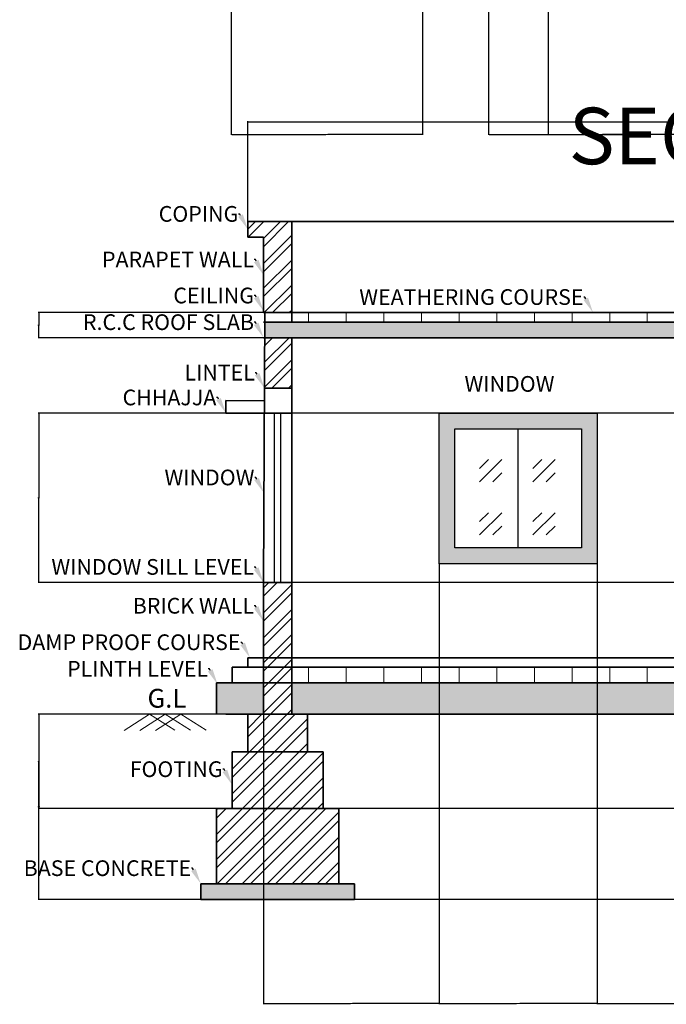
# Model space of a CAD drawing. Units: inches. Extents: x -301 to 715, y -607 to 364.
# Tile 1 of 141: x -272 to -66, y -574 to -260. Entities that reach past the tile are written whole.
import ezdxf
from ezdxf import colors
from ezdxf.entities.mleader import LeaderData, LeaderLine
from ezdxf.math import Vec2, Vec3

# ---------------------------------------------------------------- set-up
doc = ezdxf.new("R2010")
doc.units = ezdxf.units.IN
doc.header["$MEASUREMENT"] = 0
for name, color, linetype, lineweight in [('A-ANNO-DIMS', 2, 'Continuous', 18), ('A-ANNO-SYMB', 4, 'Continuous', 18), ('A-ANNO-TEXT', 4, 'Continuous', 18), ('A-ANNO-TITL', 1, 'Continuous', 35), ('A-GLAZ', 2, 'Continuous', 25), ('A-GRND', 7, 'Continuous', 25), ('A-SECT', 1, 'Continuous', 35), ('A-SECT-PATT', 8, 'Continuous', 13), ('S-FNDN', 2, 'Continuous', 35)]:
    doc.layers.add(name, color=color, linetype=linetype, lineweight=lineweight)
doc.styles.get("Standard").update_dxf_attribs({"font": 'arial.ttf'})
doc.dimstyles.get("Standard").update_dxf_attribs({"dimtxt": 0.18, "dimasz": 0.18, "dimexe": 0.18, "dimexo": 0.0625, "dimgap": 0.09, "dimtad": 0, "dimtih": 1, "dimtoh": 1, "dimdec": 1, "dimzin": 0, "dimdsep": 46, "dimlunit": 4, "dimtxsty": 'Standard', "dimcen": 0.09, "dimclrd": 3, "dimclre": 4, "dimclrt": 6, "dimadec": 0, "dimazin": 0, "dimtfac": 1, "dimtdec": 1, "dimtofl": 0, "dimtmove": 0, "dimatfit": 3, "dimfxl": 1, "dimtfill": 2, "dimtfillclr": 51, "dimtolj": 1, "dimtzin": 0, "dimarcsym": 0})

# ---------------------------------------------------------------- blocks, each defined once
blk = doc.blocks.new('GRADE-MARK-3')
for p, q in [((8.05, 5.16), (0, 0)), ((13.05, 5.16), (5, 0)), ((8.05, 5.16), (16.2, 0.15)), ((18.05, 5.16), (10, 0)), ((13.05, 5.16), (21.2, 0.15)), ((18.05, 5.16), (26.2, 0.15))]:
    blk.add_line(p, q)
blk = doc.blocks.new('*D146')
at = {"layer": 'A-ANNO-DIMS', "color": 4, "lineweight": -2, "transparency": 16777216}
for p, q in [((-204.6, -223.88), (-204.6, -296.87)), ((-143.6, -223.88), (-143.6, -296.87))]:
    blk.add_line(p, q, dxfattribs=at)
at = {"layer": 'A-ANNO-DIMS', "color": 3, "lineweight": -2, "transparency": 16777216}
for p, q in [((-204.42, -296.69), (-174.43, -296.69)), ((-143.78, -296.69), (-173.77, -296.69))]:
    blk.add_line(p, q, dxfattribs=at)
at = {"layer": 'A-ANNO-DIMS', "color": 3, "transparency": 16777216}
for points in [[(-204.42, -296.66), (-204.42, -296.72), (-204.6, -296.69)], [(-143.78, -296.66), (-143.78, -296.72), (-143.6, -296.69)]]:
    blk.add_solid(points, dxfattribs=at)
at = {"layer": 'Defpoints', "color": 0, "transparency": 16777216}
for p in [(-204.6, -223.82), (-143.6, -223.82), (-143.6, -296.69)]:
    blk.add_point(p, dxfattribs=at)
at = {"layer": 'A-ANNO-DIMS', "color": 6, "transparency": 16777216, "insert": (-174.1, -296.69), "char_height": 0.18, "attachment_point": 5, "bg_fill": 1, "box_fill_scale": 1.25, "bg_fill_color": 51, "bg_fill_transparency": 0}
blk.add_mtext('\\A1;5\'-1"', dxfattribs=at)
blk = doc.blocks.new('*D147')
at = {"layer": 'A-ANNO-DIMS', "color": 4, "lineweight": -2, "transparency": 16777216}
for p, q in [((-103.6, -223.88), (-103.6, -296.87)), ((-45.6, -223.88), (-45.6, -296.87))]:
    blk.add_line(p, q, dxfattribs=at)
at = {"layer": 'A-ANNO-DIMS', "color": 3, "lineweight": -2, "transparency": 16777216}
for p, q in [((-103.42, -296.69), (-75.01, -296.69)), ((-45.78, -296.69), (-74.2, -296.69))]:
    blk.add_line(p, q, dxfattribs=at)
at = {"layer": 'A-ANNO-DIMS', "color": 3, "transparency": 16777216}
for points in [[(-103.42, -296.66), (-103.42, -296.72), (-103.6, -296.69)], [(-45.78, -296.66), (-45.78, -296.72), (-45.6, -296.69)]]:
    blk.add_solid(points, dxfattribs=at)
at = {"layer": 'Defpoints', "color": 0, "transparency": 16777216}
for p in [(-103.6, -223.82), (-45.6, -223.82), (-45.6, -296.69)]:
    blk.add_point(p, dxfattribs=at)
at = {"layer": 'A-ANNO-DIMS', "color": 6, "transparency": 16777216, "insert": (-74.6, -296.69), "char_height": 0.18, "attachment_point": 5, "bg_fill": 1, "box_fill_scale": 1.25, "bg_fill_color": 51, "bg_fill_transparency": 0}
blk.add_mtext('\\A1;4\'-10"', dxfattribs=at)
blk = doc.blocks.new('*D158')
at = {"layer": 'A-ANNO-DIMS', "color": 4, "lineweight": -2, "transparency": 16777216}
for p, q in [((-122.6, 221.62), (-122.6, -296.87)), ((-50.6, 221.62), (-50.6, -296.87))]:
    blk.add_line(p, q, dxfattribs=at)
at = {"layer": 'A-ANNO-DIMS', "color": 3, "lineweight": -2, "transparency": 16777216}
for p, q in [((-122.42, -296.69), (-86.93, -296.69)), ((-50.78, -296.69), (-86.27, -296.69))]:
    blk.add_line(p, q, dxfattribs=at)
at = {"layer": 'A-ANNO-DIMS', "color": 3, "transparency": 16777216}
for points in [[(-122.42, -296.66), (-122.42, -296.72), (-122.6, -296.69)], [(-50.78, -296.66), (-50.78, -296.72), (-50.6, -296.69)]]:
    blk.add_solid(points, dxfattribs=at)
at = {"layer": 'Defpoints', "color": 0, "transparency": 16777216}
for p in [(-122.6, 221.68), (-50.6, 221.68), (-50.6, -296.69)]:
    blk.add_point(p, dxfattribs=at)
at = {"layer": 'A-ANNO-DIMS', "color": 6, "transparency": 16777216, "insert": (-86.6, -296.69), "char_height": 0.18, "attachment_point": 5, "bg_fill": 1, "box_fill_scale": 1.25, "bg_fill_color": 51, "bg_fill_transparency": 0}
blk.add_mtext('\\A1;6\'-0"', dxfattribs=at)
blk = doc.blocks.new('*D175')
at = {"layer": 'A-ANNO-DIMS', "color": 4, "lineweight": -2, "transparency": 16777216}
for p, q in [((-199.28, -324.41), (-199.28, -292.47)), ((148.22, -324.41), (148.22, -292.47))]:
    blk.add_line(p, q, dxfattribs=at)
at = {"layer": 'A-ANNO-DIMS', "color": 3, "lineweight": -2, "transparency": 16777216}
for p, q in [((-199.1, -292.65), (-26.21, -292.65)), ((148.04, -292.65), (-24.85, -292.65))]:
    blk.add_line(p, q, dxfattribs=at)
at = {"layer": 'A-ANNO-DIMS', "color": 3, "transparency": 16777216}
for points in [[(-199.1, -292.62), (-199.1, -292.68), (-199.28, -292.65)], [(148.04, -292.62), (148.04, -292.68), (148.22, -292.65)]]:
    blk.add_solid(points, dxfattribs=at)
at = {"layer": 'Defpoints', "color": 0, "transparency": 16777216}
for p in [(148.22, -292.65), (-199.28, -324.48), (148.22, -324.48)]:
    blk.add_point(p, dxfattribs=at)
at = {"layer": 'A-ANNO-DIMS', "color": 6, "transparency": 16777216, "insert": (-25.53, -292.65), "char_height": 0.18, "attachment_point": 5, "bg_fill": 1, "box_fill_scale": 1.25, "bg_fill_color": 51, "bg_fill_transparency": 0}
blk.add_mtext('\\A1;28\'-11 1/2"', dxfattribs=at)
blk = doc.blocks.new('*D177')
at = {"layer": 'A-ANNO-DIMS', "color": 4, "lineweight": -2, "transparency": 16777216}
for p, q in [((-138.28, -433.54), (-138.28, -573.81)), ((-194.28, -481.54), (-194.28, -573.81))]:
    blk.add_line(p, q, dxfattribs=at)
at = {"layer": 'A-ANNO-DIMS', "color": 3, "lineweight": -2, "transparency": 16777216}
for p, q in [((-194.1, -573.63), (-166.61, -573.63)), ((-138.46, -573.63), (-165.95, -573.63))]:
    blk.add_line(p, q, dxfattribs=at)
at = {"layer": 'A-ANNO-DIMS', "color": 3, "transparency": 16777216}
for points in [[(-194.1, -573.6), (-194.1, -573.66), (-194.28, -573.63)], [(-138.46, -573.6), (-138.46, -573.66), (-138.28, -573.63)]]:
    blk.add_solid(points, dxfattribs=at)
at = {"layer": 'Defpoints', "color": 0, "transparency": 16777216}
for p in [(-138.28, -433.48), (-194.28, -481.48), (-138.28, -573.63)]:
    blk.add_point(p, dxfattribs=at)
at = {"layer": 'A-ANNO-DIMS', "color": 6, "transparency": 16777216, "insert": (-166.28, -573.63), "char_height": 0.18, "attachment_point": 5, "bg_fill": 1, "box_fill_scale": 1.25, "bg_fill_color": 51, "bg_fill_transparency": 0}
blk.add_mtext('\\A1;4\'-8"', dxfattribs=at)
blk = doc.blocks.new('*D178')
at = {"layer": 'A-ANNO-DIMS', "color": 4, "lineweight": -2, "transparency": 16777216}
for p, q in [((-138.28, -433.54), (-138.28, -573.81)), ((-87.98, -433.54), (-87.98, -573.81))]:
    blk.add_line(p, q, dxfattribs=at)
at = {"layer": 'A-ANNO-DIMS', "color": 3, "lineweight": -2, "transparency": 16777216}
for p, q in [((-138.1, -573.63), (-113.67, -573.63)), ((-88.16, -573.63), (-112.59, -573.63))]:
    blk.add_line(p, q, dxfattribs=at)
at = {"layer": 'A-ANNO-DIMS', "color": 3, "transparency": 16777216}
for points in [[(-138.1, -573.6), (-138.1, -573.66), (-138.28, -573.63)], [(-88.16, -573.6), (-88.16, -573.66), (-87.98, -573.63)]]:
    blk.add_solid(points, dxfattribs=at)
at = {"layer": 'Defpoints', "color": 0, "transparency": 16777216}
for p in [(-138.28, -433.48), (-87.98, -433.48), (-87.98, -573.63)]:
    blk.add_point(p, dxfattribs=at)
at = {"layer": 'A-ANNO-DIMS', "color": 6, "transparency": 16777216, "insert": (-113.13, -573.63), "char_height": 0.18, "attachment_point": 5, "bg_fill": 1, "box_fill_scale": 1.25, "bg_fill_color": 51, "bg_fill_transparency": 0}
blk.add_mtext('\\A1;4\'-2 1/2"', dxfattribs=at)
blk = doc.blocks.new('*D179')
at = {"layer": 'A-ANNO-DIMS', "color": 4, "lineweight": -2, "transparency": 16777216}
for p, q in [((-87.98, -433.54), (-87.98, -573.81)), ((-35.28, -463.54), (-35.28, -573.81))]:
    blk.add_line(p, q, dxfattribs=at)
at = {"layer": 'A-ANNO-DIMS', "color": 3, "lineweight": -2, "transparency": 16777216}
for p, q in [((-87.8, -573.63), (-62.17, -573.63)), ((-35.46, -573.63), (-61.09, -573.63))]:
    blk.add_line(p, q, dxfattribs=at)
at = {"layer": 'A-ANNO-DIMS', "color": 3, "transparency": 16777216}
for points in [[(-87.8, -573.6), (-87.8, -573.66), (-87.98, -573.63)], [(-35.46, -573.6), (-35.46, -573.66), (-35.28, -573.63)]]:
    blk.add_solid(points, dxfattribs=at)
at = {"layer": 'Defpoints', "color": 0, "transparency": 16777216}
for p in [(-87.98, -433.48), (-35.28, -463.48), (-35.28, -573.63)]:
    blk.add_point(p, dxfattribs=at)
at = {"layer": 'A-ANNO-DIMS', "color": 6, "transparency": 16777216, "insert": (-61.63, -573.63), "char_height": 0.18, "attachment_point": 5, "bg_fill": 1, "box_fill_scale": 1.25, "bg_fill_color": 51, "bg_fill_transparency": 0}
blk.add_mtext('\\A1;4\'-4 1/2"', dxfattribs=at)
blk = doc.blocks.new('*D187')
at = {"layer": 'A-ANNO-DIMS', "color": 4, "lineweight": -2, "transparency": 16777216}
for p, q in [((139.67, -385.48), (-266.11, -385.48)), ((143.16, -439.48), (-266.11, -439.48))]:
    blk.add_line(p, q, dxfattribs=at)
at = {"layer": 'A-ANNO-DIMS', "color": 3, "lineweight": -2, "transparency": 16777216}
for p, q in [((-265.93, -385.66), (-265.93, -412.3)), ((-265.93, -439.3), (-265.93, -412.66))]:
    blk.add_line(p, q, dxfattribs=at)
at = {"layer": 'A-ANNO-DIMS', "color": 3, "transparency": 16777216}
for points in [[(-265.96, -385.66), (-265.9, -385.66), (-265.93, -385.48)], [(-265.96, -439.3), (-265.9, -439.3), (-265.93, -439.48)]]:
    blk.add_solid(points, dxfattribs=at)
at = {"layer": 'Defpoints', "color": 0, "transparency": 16777216}
for p in [(-265.93, -385.48), (139.74, -385.48), (143.22, -439.48)]:
    blk.add_point(p, dxfattribs=at)
at = {"layer": 'A-ANNO-DIMS', "color": 6, "transparency": 16777216, "insert": (-265.93, -412.48), "char_height": 0.18, "attachment_point": 5, "bg_fill": 1, "box_fill_scale": 1.25, "bg_fill_color": 51, "bg_fill_transparency": 0}
blk.add_mtext('\\A1;4\'-6"', dxfattribs=at)
blk = doc.blocks.new('*D189')
at = {"layer": 'A-ANNO-DIMS', "color": 4, "lineweight": -2, "transparency": 16777216}
for p, q in [((134.19, -353.48), (-266.11, -353.48)), ((134.19, -361.48), (-266.11, -361.48))]:
    blk.add_line(p, q, dxfattribs=at)
at = {"layer": 'A-ANNO-DIMS', "color": 3, "lineweight": -2, "transparency": 16777216}
for p, q in [((-265.93, -353.66), (-265.93, -357.3)), ((-265.93, -361.3), (-265.93, -357.66))]:
    blk.add_line(p, q, dxfattribs=at)
at = {"layer": 'A-ANNO-DIMS', "color": 3, "transparency": 16777216}
for points in [[(-265.96, -353.66), (-265.9, -353.66), (-265.93, -353.48)], [(-265.96, -361.3), (-265.9, -361.3), (-265.93, -361.48)]]:
    blk.add_solid(points, dxfattribs=at)
at = {"layer": 'Defpoints', "color": 0, "transparency": 16777216}
for p in [(134.26, -353.48), (-265.93, -361.48), (134.26, -361.48)]:
    blk.add_point(p, dxfattribs=at)
at = {"layer": 'A-ANNO-DIMS', "color": 6, "transparency": 16777216, "insert": (-265.93, -357.48), "char_height": 0.18, "attachment_point": 5, "bg_fill": 1, "box_fill_scale": 1.25, "bg_fill_color": 51, "bg_fill_transparency": 0}
blk.add_mtext('\\A1;0\'-8"', dxfattribs=at)
blk = doc.blocks.new('*D190')
at = {"layer": 'A-ANNO-DIMS', "color": 4, "lineweight": -2, "transparency": 16777216}
for p, q in [((129.19, -481.48), (-266.11, -481.48)), ((124.19, -511.48), (-266.11, -511.48))]:
    blk.add_line(p, q, dxfattribs=at)
at = {"layer": 'A-ANNO-DIMS', "color": 3, "lineweight": -2, "transparency": 16777216}
for p, q in [((-265.93, -481.66), (-265.93, -496.3)), ((-265.93, -511.3), (-265.93, -496.66))]:
    blk.add_line(p, q, dxfattribs=at)
at = {"layer": 'A-ANNO-DIMS', "color": 3, "transparency": 16777216}
for points in [[(-265.96, -481.66), (-265.9, -481.66), (-265.93, -481.48)], [(-265.96, -511.3), (-265.9, -511.3), (-265.93, -511.48)]]:
    blk.add_solid(points, dxfattribs=at)
at = {"layer": 'Defpoints', "color": 0, "transparency": 16777216}
for p in [(129.26, -481.48), (-265.93, -511.48), (124.26, -511.48)]:
    blk.add_point(p, dxfattribs=at)
at = {"layer": 'A-ANNO-DIMS', "color": 6, "transparency": 16777216, "insert": (-265.93, -496.48), "char_height": 0.18, "attachment_point": 5, "bg_fill": 1, "box_fill_scale": 1.25, "bg_fill_color": 51, "bg_fill_transparency": 0}
blk.add_mtext('\\A1;2\'-6"', dxfattribs=at)
blk = doc.blocks.new('*D191')
at = {"layer": 'A-ANNO-DIMS', "color": 4, "lineweight": -2, "transparency": 16777216}
for p, q in [((129.19, -481.48), (-266.11, -481.48)), ((114.19, -540.48), (-266.11, -540.48))]:
    blk.add_line(p, q, dxfattribs=at)
at = {"layer": 'A-ANNO-DIMS', "color": 3, "lineweight": -2, "transparency": 16777216}
for p, q in [((-265.93, -481.66), (-265.93, -510.8)), ((-265.93, -540.3), (-265.93, -511.16))]:
    blk.add_line(p, q, dxfattribs=at)
at = {"layer": 'A-ANNO-DIMS', "color": 3, "transparency": 16777216}
for points in [[(-265.96, -481.66), (-265.9, -481.66), (-265.93, -481.48)], [(-265.96, -540.3), (-265.9, -540.3), (-265.93, -540.48)]]:
    blk.add_solid(points, dxfattribs=at)
at = {"layer": 'Defpoints', "color": 0, "transparency": 16777216}
for p in [(129.26, -481.48), (-265.93, -540.48), (114.26, -540.48)]:
    blk.add_point(p, dxfattribs=at)
at = {"layer": 'A-ANNO-DIMS', "color": 6, "transparency": 16777216, "insert": (-265.93, -510.98), "char_height": 0.18, "attachment_point": 5, "bg_fill": 1, "box_fill_scale": 1.25, "bg_fill_color": 51, "bg_fill_transparency": 0}
blk.add_mtext('\\A1;4\'-11"', dxfattribs=at)

msp = doc.modelspace()

# ---------------------------------------------------------------- hatches: boundary and pattern name
at = {"layer": 'A-SECT-PATT'}
h = msp.add_hatch(dxfattribs=at)
h.set_pattern_fill('ANSI32', color=256, scale=15)
h.set_pattern_definition([(45, (10.321, 33.8764), (-3.977476, 3.977476), []), (45, (12.973, 33.8764), (-3.977476, 3.977476), [])])
h.paths.add_polyline_path([(-185.28, -324.48), (-199.28, -324.48), (-199.28, -329.48), (-194.28, -329.48), (-194.28, -353.48), (-185.28, -353.48)])
h.paths.add_polyline_path([(-185.28, -361.48), (-193.9, -361.48), (-193.98, -377.54), (-185.28, -377.54)])
h.paths.add_polyline_path([(143.22, -329.48), (148.22, -329.48), (148.22, -324.48), (134.26, -324.48), (134.26, -353.48), (143.22, -353.48)])
h.paths.add_polyline_path([(143.22, -361.48), (134.26, -361.48), (134.26, -377.48), (143.22, -377.48)])
h.paths.add_polyline_path([(-185.28, -439.48), (-194.28, -439.48), (-194.28, -463.48), (-185.28, -463.48)])
h.paths.add_polyline_path([(-185.28, -471.48), (-194.28, -471.48), (-194.28, -481.48), (-185.28, -481.48)])
h.paths.add_polyline_path([(-185.28, -463.48), (-194.28, -463.48), (-194.28, -466.48), (-185.28, -466.48)])
h.paths.add_polyline_path([(-185.28, -466.48), (-194.28, -466.48), (-194.28, -471.48), (-185.28, -471.48)])
h.paths.add_polyline_path([(-180.28, -481.48), (-185.28, -481.48), (-194.28, -481.48), (-199.28, -481.48), (-199.28, -493.48), (-180.28, -493.48)])
h.paths.add_polyline_path([(-175.28, -493.48), (-180.28, -493.48), (-199.28, -493.48), (-204.28, -493.48), (-204.28, -511.48), (-175.28, -511.48)])
h.paths.add_polyline_path([(-170.28, -511.48), (-175.28, -511.48), (-204.28, -511.48), (-209.28, -511.48), (-209.28, -535.48), (-170.28, -535.48)])
h.paths.add_polyline_path([(-35.28, -463.48), (-41.28, -463.48), (-41.28, -466.48), (-35.28, -466.48)])
h.paths.add_polyline_path([(-35.28, -466.48), (-41.28, -466.48), (-41.28, -471.48), (-35.28, -471.48)])
h.paths.add_polyline_path([(-35.28, -471.48), (-41.28, -471.48), (-41.28, -481.48), (-35.28, -481.48)])
h.paths.add_polyline_path([(-30.28, -481.48), (-46.28, -481.48), (-46.28, -493.48), (-30.28, -493.48)])
h.paths.add_polyline_path([(-25.28, -493.48), (-30.28, -493.48), (-46.28, -493.48), (-51.28, -493.48), (-51.28, -511.48), (-25.28, -511.48)])
h.paths.add_polyline_path([(-20.28, -511.48), (-25.28, -511.48), (-51.28, -511.48), (-56.28, -511.48), (-56.28, -535.48), (-20.28, -535.48)])
h.paths.add_polyline_path([(143.22, -463.48), (134.26, -463.48), (134.26, -466.48), (143.22, -466.48)])
h.paths.add_polyline_path([(143.22, -466.48), (134.26, -466.48), (134.26, -471.48), (143.22, -471.48)])
h.paths.add_polyline_path([(143.22, -471.48), (134.26, -471.48), (134.26, -481.48), (143.22, -481.48)])
h.paths.add_polyline_path([(148.26, -481.48), (143.26, -481.48), (134.26, -481.48), (129.26, -481.48), (129.26, -493.48), (148.26, -493.48)])
h.paths.add_polyline_path([(153.26, -493.48), (148.26, -493.48), (129.26, -493.48), (124.26, -493.48), (124.26, -511.48), (153.26, -511.48)])
h.paths.add_polyline_path([(158.26, -511.48), (153.26, -511.48), (124.26, -511.48), (119.26, -511.48), (119.26, -535.48), (158.26, -535.48)])
h = msp.add_hatch(dxfattribs=at)
h.set_pattern_fill('ANSI31', color=256, scale=96, angle=45, style=0)
h.paths.add_polyline_path([(-185.28, -356.48), (134.26, -356.48), (134.26, -353.48), (-185.28, -353.48)])
h = msp.add_hatch(dxfattribs=at)
h.set_pattern_fill('AR-CONC', color=256, scale=0.5)
h.set_pattern_definition([(50, (10.3213, 33.8764), (3.586301, -0.31376), [0.375, -4.125]), (355, (10.3213, 33.8764), (-0.693757, 3.76096), [0.3, -3.3]), (100.45144, (10.62, 33.8502), (2.892544, 3.4472), [0.3187, -3.50571]), (46.1842, (10.3213, 34.8764), (5.336207, -0.827596), [0.5625, -6.1875]), (96.6356, (10.766, 34.8074), (4.67331, 4.870593), [0.47805, -5.25857]), (351.1842, (10.321, 34.8764), (4.67331, 4.870593), [0.45, -4.95]), (21, (10.8213, 34.6264), (2.984535, -2.013094), [0.375, -4.125]), (326, (10.8213, 34.6264), (1.216577, 3.62575), [0.3, -3.3]), (71.45144, (11.07, 34.4586), (4.201112, 1.612656), [0.3187, -3.50571]), (37.5, (10.3213, 33.8764), (0.0607993, 1.6644693), [0, -3.26, 0, -3.35, 0, -3.3125]), (7.5, (10.3213, 33.8764), (1.3153477, 1.9720586), [0, -1.91, 0, -3.185, 0, -1.2625]), (327.5, (9.2063, 33.8764), (2.6691122, -0.1127744), [0, -1.25, 0, -3.9, 0, -5.175]), (317.5, (8.7063, 33.8764), (2.915931, 0.500525), [0, -1.625, 0, -2.59, 0, -3.675])])
h.paths.add_polyline_path([(-56.28, -535.48), (-61.28, -535.48), (-61.28, -540.48), (-15.28, -540.48), (-15.28, -535.48), (-20.28, -535.48)])
h.paths.add_polyline_path([(119.26, -535.48), (114.26, -535.48), (114.26, -540.48), (163.26, -540.48), (163.26, -535.48), (158.26, -535.48)])
h.paths.add_polyline_path([(-206.28, -471.48), (-209.28, -471.48), (-209.28, -481.48), (-206.28, -481.48), (-194.28, -481.48), (-194.28, -471.48)])
h.paths.add_polyline_path([(-41.28, -481.48), (-41.28, -471.48), (-185.28, -471.48), (-185.28, -481.48), (-180.28, -481.48)])
h.paths.add_polyline_path([(134.26, -481.48), (134.26, -471.48), (-35.28, -471.48), (-35.28, -481.48), (-30.28, -481.48)])
h.paths.add_polyline_path([(155.22, -481.48), (158.22, -481.48), (158.22, -471.48), (153.22, -471.48), (143.22, -471.48), (143.22, -481.48), (148.26, -481.48)])
h.paths.add_polyline_path([(-193.88, -356.48), (-193.9, -361.48), (143.22, -361.48), (143.22, -356.48)])
h = msp.add_hatch(color=256, dxfattribs=at)
h.dxf.hatch_style = 1
h.paths.add_polyline_path([(-138.28, -385.48), (-138.28, -433.48), (-87.98, -433.48), (-87.98, -385.48)])
h.paths.add_polyline_path([(-92.98, -390.48), (-92.98, -428.48), (-133.28, -428.48), (-133.28, -390.48)], flags=16)
h.paths.add_polyline_path([(-35.28, -385.48), (-35.28, -463.48), (12.72, -463.48), (12.72, -385.48)])
h.paths.add_polyline_path([(-30.28, -390.48), (7.72, -390.48), (7.72, -458.48), (-30.28, -458.48)], flags=16)
h.paths.add_polyline_path([(48.47, -385.48), (48.47, -433.48), (98.47, -433.48), (98.47, -385.48)])
h.paths.add_polyline_path([(93.47, -390.48), (93.47, -428.48), (53.47, -428.48), (53.47, -390.48)], flags=16)
h = msp.add_hatch(dxfattribs=at)
h.set_pattern_fill('GOST_GLASS', color=256, scale=2)
h.set_pattern_definition([(45, (10.321, 33.876), (16.97056, -2e-15), [10, -14]), (45, (14.564, 33.876), (16.97056, -2e-15), [4, -20]), (45, (10.321, 38.119), (16.97056, -2e-15), [4, -20])])
h.paths.add_polyline_path([(-113.13, -390.48), (-133.28, -390.48), (-133.28, -428.48), (-113.13, -428.48)])
h.paths.add_polyline_path([(-92.98, -390.48), (-113.13, -390.48), (-113.13, -428.48), (-92.98, -428.48)])
h.paths.add_polyline_path([(73.47, -390.48), (53.47, -390.48), (53.47, -428.48), (73.47, -428.48)])
h.paths.add_polyline_path([(93.47, -390.48), (73.47, -390.48), (73.47, -428.48), (93.47, -428.48)])
h = msp.add_hatch(dxfattribs=at)
h.set_pattern_fill('ANSI31', color=256, scale=96, angle=45, style=0)
h.paths.add_polyline_path([(-185.28, -471.48), (-41.28, -471.48), (-41.28, -466.48), (-185.28, -466.48)])
h = msp.add_hatch(dxfattribs=at)
h.set_pattern_fill('AR-CONC', color=256, scale=0.25)
h.set_pattern_definition([(50, (10.3213, 33.8764), (1.7931505, -0.1568803), [0.1875, -2.0625]), (355, (10.3213, 33.8764), (-0.3468783, 1.8804803), [0.15, -1.65]), (100.45144, (10.4707, 33.8633), (1.446272, 1.7236), [0.1593505, -1.7528553]), (46.1842, (10.3213, 34.3764), (2.668103, -0.413798), [0.28125, -3.09375]), (96.63564, (10.5436, 34.342), (2.336655, 2.435297), [0.239026, -2.629284]), (351.18416, (10.3213, 34.3764), (2.336655, 2.435297), [0.225, -2.475]), (21, (10.5713, 34.2514), (1.4922676, -1.0065472), [0.1875, -2.0625]), (326, (10.5713, 34.2514), (0.6082883, 1.812875), [0.15, -1.65]), (71.45144, (10.6956, 34.1675), (2.100556, 0.806328), [0.1593505, -1.7528553]), (37.5, (10.3213, 33.8764), (0.03039964, 0.83223463), [0, -1.63, 0, -1.675, 0, -1.65625]), (7.5, (10.3213, 33.8764), (0.6576738, 0.9860293), [0, -0.955, 0, -1.5925, 0, -0.63125]), (327.5, (9.7638, 33.8764), (1.3345561, -0.0563872), [0, -0.625, 0, -1.95, 0, -2.5875]), (317.5, (9.5138, 33.8764), (1.4579654, 0.2502625), [0, -0.8125, 0, -1.295, 0, -1.8375])])
h.paths.add_polyline_path([(-165.28, -540.48), (-165.28, -535.48), (-170.28, -535.48), (-209.28, -535.48), (-214.28, -535.48), (-214.28, -540.48)])

# ---------------------------------------------------------------- linework, layer by layer
at = {"layer": 'A-GLAZ'}
for p, q in [((-190.78, -439.48), (-190.78, -385.48)), ((-188.78, -439.48), (-188.78, -385.48)), ((-113.13, -428.48), (-113.13, -390.48))]:
    msp.add_line(p, q, dxfattribs=at)
for points in [[(-138.28, -385.48), (-87.98, -385.48), (-87.98, -433.48), (-138.28, -433.48)], [(-133.28, -390.48), (-92.98, -390.48), (-92.98, -428.48), (-133.28, -428.48)]]:
    msp.add_lwpolyline(points, close=True, dxfattribs=at)
at = {"layer": 'A-GRND'}
for q in [(-242.28, -481.48), (155.22, -481.48)]:
    msp.add_line((-206.28, -481.48), q, dxfattribs=at)
at = {"layer": 'A-SECT'}
for p, q in [((-199.28, -329.48), (-199.28, -324.48)), ((-199.28, -324.48), (-185.28, -324.48)), ((-185.28, -324.48), (-185.28, -353.48)), ((-185.28, -324.48), (134.26, -324.48)), ((-194.28, -329.48), (-199.28, -329.48)), ((-194.28, -353.48), (-194.28, -329.48)), ((-193.87, -353.48), (-194.28, -439.48)), ((-194.28, -353.48), (143.22, -353.48)), ((-185.28, -353.48), (-185.28, -356.48)), ((-194.28, -356.48), (143.22, -356.48)), ((-194.28, -361.48), (143.22, -361.48)), ((-185.28, -361.48), (-185.28, -439.48)), ((-194, -381.54), (-194, -377.54)), ((-194, -377.54), (-185.28, -377.54)), ((-206.28, -383.48), (-206.28, -381.48)), ((-206.28, -381.48), (-194, -381.54)), ((-206.28, -385.48), (-206.28, -383.48)), ((-206.28, -385.48), (-185.28, -385.48)), ((-194.28, -481.48), (-194.28, -439.48)), ((-194.28, -439.48), (-185.28, -439.48)), ((-185.28, -439.48), (-185.28, -481.48)), ((-194.28, -463.48), (-199.28, -463.48)), ((-199.28, -463.48), (-199.28, -466.48)), ((-199.28, -463.48), (148.26, -463.48)), ((-204.28, -466.48), (153.22, -466.48)), ((-199.28, -466.48), (-204.28, -466.48)), ((-204.28, -466.48), (-204.28, -471.48)), ((-185.28, -466.48), (-185.28, -471.48)), ((-204.28, -471.48), (-209.28, -471.48)), ((-209.28, -471.48), (-209.28, -481.48)), ((-206.28, -471.48), (155.22, -471.48))]:
    msp.add_line(p, q, dxfattribs=at)
at = {"layer": 'S-FNDN'}
for p, q in [((-194.28, -481.48), (-199.28, -481.48)), ((-199.28, -481.48), (-199.28, -493.48)), ((-185.28, -481.48), (-180.28, -481.48)), ((-180.28, -481.48), (-180.28, -493.48)), ((-199.28, -493.48), (-204.28, -493.48)), ((-204.28, -493.48), (-204.28, -511.48)), ((-199.28, -493.48), (-180.28, -493.48)), ((-180.28, -493.48), (-175.28, -493.48)), ((-175.28, -493.48), (-175.28, -511.48)), ((-204.28, -511.48), (-209.28, -511.48)), ((-209.28, -511.48), (-209.28, -535.48)), ((-204.28, -511.48), (-175.28, -511.48)), ((-175.28, -511.48), (-170.28, -511.48)), ((-170.28, -511.48), (-170.28, -535.48)), ((-209.28, -535.48), (-214.28, -535.48)), ((-214.28, -535.48), (-214.28, -540.48)), ((-209.28, -535.48), (-170.28, -535.48)), ((-170.28, -535.48), (-165.28, -535.48)), ((-165.28, -535.48), (-165.28, -540.48)), ((-214.28, -540.48), (-165.28, -540.48))]:
    msp.add_line(p, q, dxfattribs=at)

# ---------------------------------------------------------------- block references
at = {"layer": 'A-ANNO-SYMB'}
msp.add_blockref('GRADE-MARK-3', (-238.72, -486.64), dxfattribs=at)

# ---------------------------------------------------------------- texts
msp.add_text('G.L', height=6, dxfattribs=at).set_placement((-231.26, -479.37))
at = {"layer": 'A-ANNO-TEXT', "insert": (-130.25, -373.68), "char_height": 5, "attachment_point": 1}
msp.add_mtext_dynamic_manual_height_columns('WINDOW', width=73.06, gutter_width=1, heights=[0], dxfattribs=at)
at = {"layer": 'A-ANNO-TITL'}
msp.add_text('SECTION', height=18, dxfattribs=at).set_placement((-97.05, -306.18))

# ---------------------------------------------------------------- dimensions: what is measured, and where the dimension line sits
at = {"layer": 'A-ANNO-DIMS'}
for base, p1, p2, picture, middle in [((-50.6, -296.69), (-122.6, 221.68), (-50.6, 221.68), '*D158', (-86.6, -296.69)), ((-143.6, -296.69), (-204.6, -223.82), (-143.6, -223.82), '*D146', (-174.1, -296.69)), ((-45.6, -296.69), (-103.6, -223.82), (-45.6, -223.82), '*D147', (-74.6, -296.69)), ((148.22, -292.65), (-199.28, -324.48), (148.22, -324.48), '*D175', (-25.53, -292.65)), ((-138.28, -573.63), (-194.28, -481.48), (-138.28, -433.48), '*D177', (-166.28, -573.63)), ((-87.98, -573.63), (-138.28, -433.48), (-87.98, -433.48), '*D178', (-113.13, -573.63)), ((-35.28, -573.63), (-87.98, -433.48), (-35.28, -463.48), '*D179', (-61.63, -573.63))]:
    dim = msp.add_linear_dim(base=base, p1=p1, p2=p2, dimstyle='Standard', override={"dimdec": 1, "dimlfac": 1, "dimrnd": 0, "dimzin": 1, "dimdsep": 46, "dimlunit": 4, "dimfrac": 2}, dxfattribs=at)
    dim.commit()
    dim.dimension.update_dxf_attribs({"geometry": picture, "text_midpoint": middle})
for base, p1, p2, picture, middle in [((-265.93, -361.48), (134.26, -353.48), (134.26, -361.48), '*D189', (-265.93, -357.48)), ((-265.93, -385.48), (143.22, -439.48), (139.74, -385.48), '*D187', (-265.93, -412.48)), ((-265.93, -540.48), (129.26, -481.48), (114.26, -540.48), '*D191', (-265.93, -510.98)), ((-265.93, -511.48), (129.26, -481.48), (124.26, -511.48), '*D190', (-265.93, -496.48))]:
    dim = msp.add_linear_dim(base=base, p1=p1, p2=p2, angle=90, dimstyle='Standard', override={"dimdec": 1, "dimlfac": 1, "dimrnd": 0, "dimzin": 1, "dimdsep": 46, "dimlunit": 4, "dimfrac": 2}, dxfattribs=at)
    dim.commit()
    dim.dimension.update_dxf_attribs({"geometry": picture, "text_midpoint": middle})

# ---------------------------------------------------------------- leaders
at = {"layer": 'A-ANNO-TEXT'}
ml = msp.add_multileader_mtext('Standard', dxfattribs=at)
ml.set_content('COPING', color=256)
ml.set_leader_properties()
ml.build(insert=Vec2(0, 0))
ml.multileader.update_dxf_attribs({"dogleg_length": 0.36, "arrow_head_size": 5})
ctx = ml.context
ctx.base_point, ctx.char_height, ctx.arrow_head_size, ctx.landing_gap_size, ctx.plane_origin = Vec3(-229.19, -322.05), 5, 5, 0.09, Vec3(-199.28, -326.98)
ctx.text_align_type = 2
notes = []
notes.append((ctx, [(0, (1, 1, 0), (-201.88, -322.05), (-1, 0), 0.36, [(0, [(-199.28, -326.98)], 0, [])])]))
ctx.mtext.insert, ctx.mtext.alignment, ctx.mtext.flow_direction = Vec3(-202.33, -319.51), 3, 5
ml = msp.add_multileader_mtext('Standard', dxfattribs=at)
ml.set_content('PARAPET WALL', color=256)
ml.set_leader_properties()
ml.build(insert=Vec2(0, 0))
ml.multileader.update_dxf_attribs({"dogleg_length": 0.36, "arrow_head_size": 5})
ctx = ml.context
ctx.base_point, ctx.char_height, ctx.arrow_head_size, ctx.landing_gap_size, ctx.plane_origin = Vec3(-250.2, -336.55), 5, 5, 0.09, Vec3(-194.28, -341.48)
ctx.text_align_type = 2
notes.append((ctx, [(0, (1, 1, 0), (-196.88, -336.55), (-1, 0), 0.36, [(0, [(-194.28, -341.48)], 0, [])])]))
ctx.mtext.insert, ctx.mtext.alignment, ctx.mtext.flow_direction = Vec3(-197.33, -334.05), 3, 5
ml = msp.add_multileader_mtext('Standard', dxfattribs=at)
ml.set_content('CEILING', color=256)
ml.set_leader_properties()
ml.build(insert=Vec2(0, 0))
ml.multileader.update_dxf_attribs({"dogleg_length": 0.36, "arrow_head_size": 5})
ctx = ml.context
ctx.base_point, ctx.char_height, ctx.arrow_head_size, ctx.landing_gap_size, ctx.plane_origin = Vec3(-224.58, -348.06), 5, 5, 0.09, Vec3(-194.28, -352.99)
ctx.text_align_type = 2
notes.append((ctx, [(0, (1, 1, 0), (-196.88, -348.06), (-1, 0), 0.36, [(0, [(-194.28, -352.99)], 0, [])])]))
ctx.mtext.insert, ctx.mtext.alignment, ctx.mtext.flow_direction = Vec3(-197.33, -345.52), 3, 5
ml = msp.add_multileader_mtext('Standard', dxfattribs=at)
ml.set_content('WEATHERING COURSE', color=256)
ml.set_leader_properties()
ml.build(insert=Vec2(0, 0))
ml.multileader.update_dxf_attribs({"dogleg_length": 0.36, "arrow_head_size": 5})
ctx = ml.context
ctx.base_point, ctx.char_height, ctx.arrow_head_size, ctx.landing_gap_size, ctx.plane_origin = Vec3(-171.13, -348.55), 5, 5, 0.09, Vec3(-89.28, -353.48)
ctx.text_align_type = 2
notes.append((ctx, [(0, (1, 1, 0), (-91.88, -348.55), (-1, 0), 0.36, [(0, [(-89.28, -353.48)], 0, [])])]))
ctx.mtext.insert, ctx.mtext.alignment, ctx.mtext.flow_direction = Vec3(-92.33, -346.01), 3, 5
ml = msp.add_multileader_mtext('Standard', dxfattribs=at)
ml.set_content('R.C.C ROOF SLAB', color=256)
ml.set_leader_properties()
ml.build(insert=Vec2(0, 0))
ml.multileader.update_dxf_attribs({"dogleg_length": 0.36, "arrow_head_size": 5})
ctx = ml.context
ctx.base_point, ctx.char_height, ctx.arrow_head_size, ctx.landing_gap_size, ctx.plane_origin = Vec3(-257.43, -356.55), 5, 5, 0.09, Vec3(-194.28, -361.48)
ctx.text_align_type = 2
notes.append((ctx, [(0, (1, 1, 0), (-196.88, -356.55), (-1, 0), 0.36, [(0, [(-194.28, -361.48)], 0, [])])]))
ctx.mtext.insert, ctx.mtext.alignment, ctx.mtext.flow_direction = Vec3(-197.33, -354.01), 3, 5
ml = msp.add_multileader_mtext('Standard', dxfattribs=at)
ml.set_content('LINTEL', color=256)
ml.set_leader_properties()
ml.build(insert=Vec2(0, 0))
ml.multileader.update_dxf_attribs({"dogleg_length": 0.36, "arrow_head_size": 5})
ctx = ml.context
ctx.base_point, ctx.char_height, ctx.arrow_head_size, ctx.landing_gap_size, ctx.plane_origin = Vec3(-220.06, -372.61), 5, 5, 0.09, Vec3(-194, -377.54)
ctx.text_align_type = 2
notes.append((ctx, [(0, (1, 1, 0), (-196.6, -372.61), (-1, 0), 0.36, [(0, [(-194, -377.54)], 0, [])])]))
ctx.mtext.insert, ctx.mtext.alignment, ctx.mtext.flow_direction = Vec3(-197.05, -370.11), 3, 5
ml = msp.add_multileader_mtext('Standard', dxfattribs=at)
ml.set_content('CHHAJJA', color=256)
ml.set_leader_properties()
ml.build(insert=Vec2(0, 0))
ml.multileader.update_dxf_attribs({"dogleg_length": 0.36, "arrow_head_size": 5})
ctx = ml.context
ctx.base_point, ctx.char_height, ctx.arrow_head_size, ctx.landing_gap_size, ctx.plane_origin = Vec3(-240.52, -380.55), 5, 5, 0.09, Vec3(-206.28, -385.48)
ctx.text_align_type = 2
notes.append((ctx, [(0, (1, 1, 0), (-208.88, -380.55), (-1, 0), 0.36, [(0, [(-206.28, -385.48)], 0, [])])]))
ctx.mtext.insert, ctx.mtext.alignment, ctx.mtext.flow_direction = Vec3(-209.33, -378.01), 3, 5
ml = msp.add_multileader_mtext('Standard', dxfattribs=at)
ml.set_content('WINDOW', color=256)
ml.set_leader_properties()
ml.build(insert=Vec2(0, 0))
ml.multileader.update_dxf_attribs({"dogleg_length": 0.36, "arrow_head_size": 5})
ctx = ml.context
ctx.base_point, ctx.char_height, ctx.arrow_head_size, ctx.landing_gap_size, ctx.plane_origin = Vec3(-227.77, -406.05), 5, 5, 0.09, Vec3(-194.14, -410.97)
ctx.text_align_type = 2
notes.append((ctx, [(0, (1, 1, 0), (-196.74, -406.05), (-1, 0), 0.36, [(0, [(-194.14, -410.97)], 0, [])])]))
ctx.mtext.insert, ctx.mtext.alignment, ctx.mtext.flow_direction = Vec3(-197.19, -403.5), 3, 5
ml = msp.add_multileader_mtext('Standard', dxfattribs=at)
ml.set_content('WINDOW SILL LEVEL', color=256)
ml.set_leader_properties()
ml.build(insert=Vec2(0, 0))
ml.multileader.update_dxf_attribs({"dogleg_length": 0.36, "arrow_head_size": 5})
ctx = ml.context
ctx.base_point, ctx.char_height, ctx.arrow_head_size, ctx.landing_gap_size, ctx.plane_origin = Vec3(-267.73, -434.55), 5, 5, 0.09, Vec3(-194.28, -439.48)
ctx.text_align_type = 2
notes.append((ctx, [(0, (1, 1, 0), (-196.88, -434.55), (-1, 0), 0.36, [(0, [(-194.28, -439.48)], 0, [])])]))
ctx.mtext.insert, ctx.mtext.alignment, ctx.mtext.flow_direction = Vec3(-197.33, -432.01), 3, 5
ml = msp.add_multileader_mtext('Standard', dxfattribs=at)
ml.set_content('BRICK WALL', color=256)
ml.set_leader_properties()
ml.build(insert=Vec2(0, 0))
ml.multileader.update_dxf_attribs({"dogleg_length": 0.36, "arrow_head_size": 5})
ctx = ml.context
ctx.base_point, ctx.char_height, ctx.arrow_head_size, ctx.landing_gap_size, ctx.plane_origin = Vec3(-238.97, -446.93), 5, 5, 0.09, Vec3(-194.28, -451.86)
ctx.text_align_type = 2
notes.append((ctx, [(0, (1, 1, 0), (-196.88, -446.93), (-1, 0), 0.36, [(0, [(-194.28, -451.86)], 0, [])])]))
ctx.mtext.insert, ctx.mtext.alignment, ctx.mtext.flow_direction = Vec3(-197.33, -444.39), 3, 5
ml = msp.add_multileader_mtext('Standard', dxfattribs=at)
ml.set_content('DAMP PROOF COURSE', color=256)
ml.set_leader_properties()
ml.build(insert=Vec2(0, 0))
ml.multileader.update_dxf_attribs({"dogleg_length": 0.36, "arrow_head_size": 5})
ctx = ml.context
ctx.base_point, ctx.char_height, ctx.arrow_head_size, ctx.landing_gap_size, ctx.plane_origin = Vec3(-279.6, -458.55), 5, 5, 0.09, Vec3(-198.6, -463.48)
ctx.text_align_type = 2
notes.append((ctx, [(0, (1, 1, 0), (-201.2, -458.55), (-1, 0), 0.36, [(0, [(-198.6, -463.48)], 0, [])])]))
ctx.mtext.insert, ctx.mtext.alignment, ctx.mtext.flow_direction = Vec3(-201.65, -456.01), 3, 5
ml = msp.add_multileader_mtext('Standard', dxfattribs=at)
ml.set_content('PLINTH LEVEL', color=256)
ml.set_leader_properties()
ml.build(insert=Vec2(0, 0))
ml.multileader.update_dxf_attribs({"dogleg_length": 0.36, "arrow_head_size": 5})
ctx = ml.context
ctx.base_point, ctx.char_height, ctx.arrow_head_size, ctx.landing_gap_size, ctx.plane_origin = Vec3(-259.82, -466.98), 5, 5, 0.09, Vec3(-208.94, -471.91)
ctx.text_align_type = 2
notes.append((ctx, [(0, (1, 1, 0), (-211.54, -466.98), (-1, 0), 0.36, [(0, [(-208.94, -471.91)], 0, [])])]))
ctx.mtext.insert, ctx.mtext.alignment, ctx.mtext.flow_direction = Vec3(-211.99, -464.48), 3, 5
ml = msp.add_multileader_mtext('Standard', dxfattribs=at)
ml.set_content('FOOTING', color=256)
ml.set_leader_properties()
ml.build(insert=Vec2(0, 0))
ml.multileader.update_dxf_attribs({"dogleg_length": 0.36, "arrow_head_size": 5})
ctx = ml.context
ctx.base_point, ctx.char_height, ctx.arrow_head_size, ctx.landing_gap_size, ctx.plane_origin = Vec3(-238.23, -499), 5, 5, 0.09, Vec3(-204.28, -503.93)
ctx.text_align_type = 2
notes.append((ctx, [(0, (1, 1, 0), (-206.88, -499), (-1, 0), 0.36, [(0, [(-204.28, -503.93)], 0, [])])]))
ctx.mtext.insert, ctx.mtext.alignment, ctx.mtext.flow_direction = Vec3(-207.33, -496.46), 3, 5
ml = msp.add_multileader_mtext('Standard', dxfattribs=at)
ml.set_content('{\\C256;\\c16777215;BASE CONCRETE}', color=256)
ml.set_leader_properties()
ml.build(insert=Vec2(0, 0))
ml.multileader.update_dxf_attribs({"dogleg_length": 0.36, "arrow_head_size": 5})
ctx = ml.context
ctx.base_point, ctx.char_height, ctx.arrow_head_size, ctx.landing_gap_size, ctx.plane_origin = Vec3(-276.3, -530.55), 5, 5, 0.09, Vec3(-214.28, -535.48)
ctx.text_align_type = 2
notes.append((ctx, [(0, (1, 1, 0), (-216.88, -530.55), (-1, 0), 0.36, [(0, [(-214.28, -535.48)], 0, [])])]))
ctx.mtext.insert, ctx.mtext.alignment, ctx.mtext.flow_direction = Vec3(-217.33, -528.01), 3, 5
for ctx, leaders in notes:
    for number, flags, end, landing, length, lines in leaders:
        leader = LeaderData()
        leader.index, (leader.has_last_leader_line, leader.has_dogleg_vector, leader.attachment_direction) = number, flags
        leader.last_leader_point, leader.dogleg_vector, leader.dogleg_length = Vec3(end), Vec3(landing), length
        for number, points, colour, breaks in lines:
            line = LeaderLine()
            line.index, line.vertices, line.color, line.breaks = number, Vec3.list(points), colors.encode_raw_color(colour), breaks
            leader.lines.append(line)
        ctx.leaders.append(leader)

doc.saveas('drawing.dxf')
